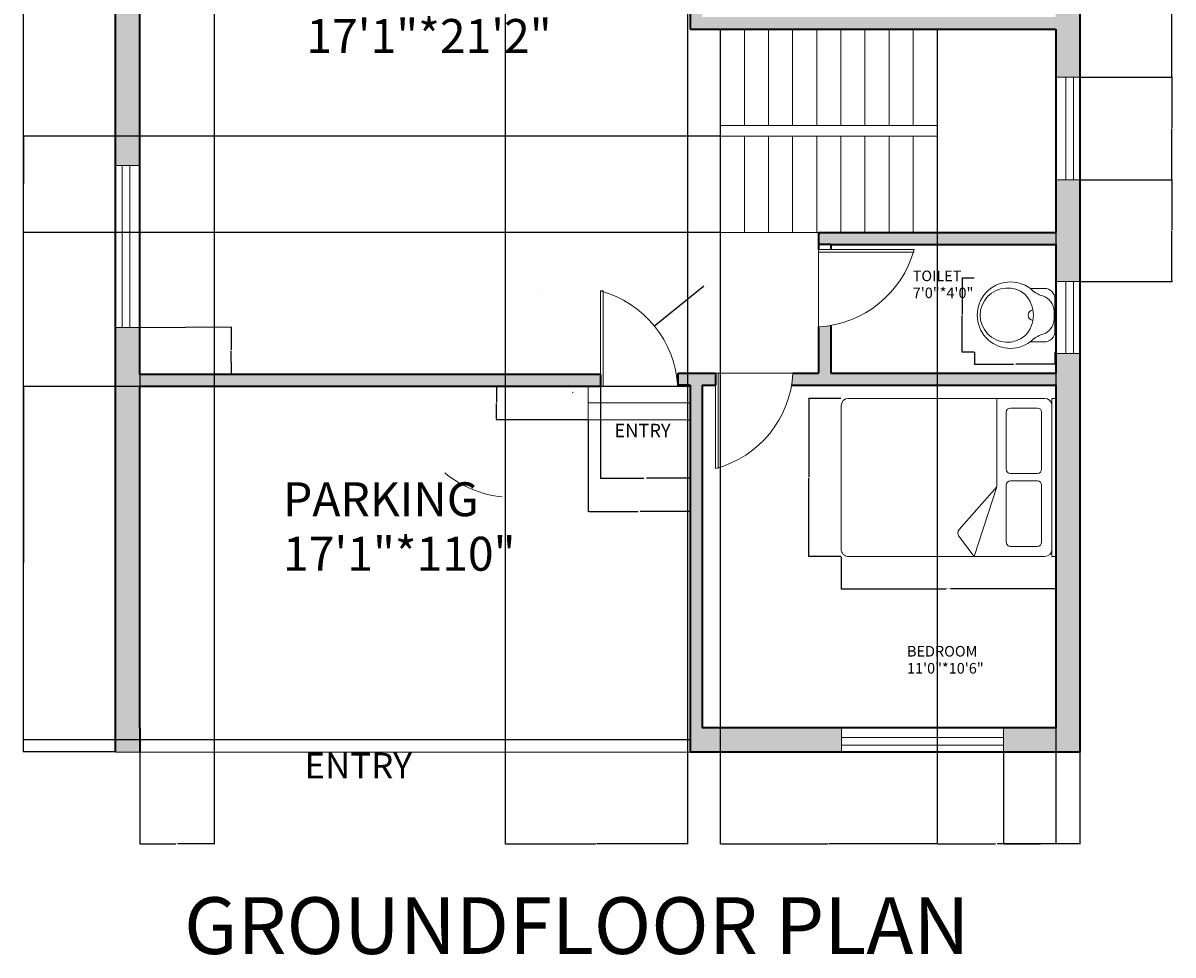
# Model space of a CAD drawing. Units: feet. Extents: x 2516 to 2945, y 1283 to 1993.
# Tile 1 of 3: x 2516 to 2945, y 1283 to 1631. Entities that reach past the tile are written whole.
import ezdxf

# ---------------------------------------------------------------- set-up
doc = ezdxf.new("R2010")
doc.units = ezdxf.units.FT
doc.layers.get('0').update_dxf_attribs({"lineweight": 18})
for name, color, linetype, lineweight in [('A-ANNO-DIMS', 2, 'Continuous', 18), ('A-ANNO-TEXT', 7, 'Continuous', 18), ('A-AREA-IDEN', 7, 'Continuous', 18), ('A-FLOR', 221, 'Continuous', 18), ('A-FLOR-FIXT', 8, 'Continuous', 18), ('A-FLOR-STRS', 7, 'Continuous', 18), ('A-FURN', 8, 'Continuous', 18), ('A-WALL', 7, 'Continuous', 35), ('A-WALL-PATT', 143, 'Continuous', 13), ('doors', 163, 'Continuous', 18), ('windows', 10, 'Continuous', 18)]:
    doc.layers.add(name, color=color, linetype=linetype, lineweight=lineweight)
doc.styles.get("Standard").update_dxf_attribs({"font": 'arial.ttf'})
doc.dimstyles.get("Standard").update_dxf_attribs({"dimtxt": 0.18, "dimasz": 0.18, "dimexe": 0.18, "dimexo": 0.0625, "dimgap": 0.09, "dimtad": 0, "dimtih": 1, "dimtoh": 1, "dimdec": 4, "dimzin": 0, "dimdsep": 46, "dimtxsty": 'Standard', "dimcen": 0.09, "dimadec": 0, "dimazin": 0, "dimtfac": 1, "dimtdec": 4, "dimtofl": 0, "dimtmove": 0, "dimatfit": 3, "dimfxl": 1, "dimtolj": 1, "dimtzin": 0, "dimarcsym": 0})

# ---------------------------------------------------------------- blocks, each defined once
blk = doc.blocks.new('door')
at = {"layer": 'doors'}
for p, q in [((-0.98, 0), (-0.98, 35.67)), ((0, 35.67), (0, 0)), ((-0.98, 0), (27.91, 0))]:
    blk.add_line(p, q, dxfattribs=at)
blk.add_arc((-11.23, -2.17), 39.2, 3.167, 74.8469, dxfattribs=at)
blk = doc.blocks.new('A$C6EF51710')
at = {"linetype": 'ByBlock'}
for p, q in [((0.0508, 0.2843), (0.1169, 0.2843)), ((0, 0.0811), (0, 0.2335)), ((0.0041, 0.1392), (0.0041, 0.1755)), ((0.1169, 0.0303), (0.0508, 0.0303))]:
    blk.add_line(p, q, dxfattribs=at)
for centre, radius, start, end in [((0.0508, 0.2335), 0.0508, 90, 180), ((0.0168, 0.3818), 0.1397, 287.1046, 315), ((0.2107, 0.1573), 0.1576, 232.8984, 127.1016), ((0.2254, 0.1573), 0.1289, 230.0084, 129.9916), ((0.0803, 0.1755), 0.0762, 107.1046, 180), ((0.2413, 0.1573), 0.1397, 135, 225), ((0.1016, 0.1573), 0.0254, 275.2159, 84.7841), ((0.0803, 0.1392), 0.0762, 180, 252.8954), ((0.0508, 0.0811), 0.0508, 180, 270), ((0.0168, -0.0672), 0.1397, 45, 72.8954)]:
    blk.add_arc(centre, radius, start, end, dxfattribs=at)
blk = doc.blocks.new('A$C03A44EBA')
at = {"rotation": 270}
blk.add_blockref('A$C6EF51710', (0.0003, 0.3683), dxfattribs=at)
blk = doc.blocks.new('A$C164346CA')
for p, q in [((0, 2.035), (0, 2)), ((1.5, 2.035), (0, 2.035)), ((1.5, 2), (0, 2)), ((1.5, 2), (1.5, 2.035)), ((0, 1.93), (0, 0.07)), ((0.092, 1.862), (0.092, 1.607)), ((0.673, 1.902), (0.132, 1.902)), ((0.713, 1.607), (0.713, 1.862)), ((0.783, 1.862), (0.783, 1.607)), ((1.364, 1.902), (0.823, 1.902)), ((1.404, 1.607), (1.404, 1.862)), ((1.5, 0.07), (1.5, 1.93)), ((0.132, 1.567), (0.673, 1.567)), ((0.823, 1.567), (1.364, 1.567)), ((0.839, 1.476), (0, 1.476)), ((0.839, 1.476), (1.245, 1.12)), ((1.5, 1.261), (0.839, 1.476)), ((1.308, 1.117), (1.5, 1.261)), ((0.07, 0), (1.43, 0))]:
    blk.add_line(p, q)
for centre, radius, start, end in [((0.07, 1.93), 0.07, 90, 180), ((1.43, 1.93), 0.07, 0, 90), ((0.132, 1.862), 0.04, 90, 180), ((0.673, 1.862), 0.04, 0, 90), ((0.823, 1.862), 0.04, 90, 180), ((1.364, 1.862), 0.04, 0, 90), ((0.132, 1.607), 0.04, 180, 270), ((0.673, 1.607), 0.04, 270, 0), ((0.823, 1.607), 0.04, 180, 270), ((1.364, 1.607), 0.04, 270, 0), ((1.278, 1.158), 0.05, 228.6958, 306.7579), ((0.07, 0.07), 0.07, 180, 270), ((1.43, 0.07), 0.07, 270, 0)]:
    blk.add_arc(centre, radius, start, end)
blk = doc.blocks.new('WIN-STANDARD')
for p, q in [((2.52, 60.52), (2.52, 0)), ((5.4, 60.52), (5.4, 0))]:
    blk.add_line(p, q)
blk.add_lwpolyline([(0, 60.52), (9, 60.52), (9, 0), (0, 0)], close=True)
blk = doc.blocks.new('WIN-TOILET')
for p, q in [((0, 5.4), (26.87, 5.4)), ((0, 2.52), (26.87, 2.52))]:
    blk.add_line(p, q)
blk.add_lwpolyline([(0, 9), (26.87, 9), (26.87, 0), (0, 0)], close=True)
blk = doc.blocks.new('*D17')
at = {"layer": 'A-ANNO-DIMS', "color": 0, "lineweight": -2, "transparency": 16777216}
for p, q in [((2821.29, 1431.8), (2821.29, 1419.66)), ((2901.42, 1431.8), (2901.42, 1419.66)), ((2821.47, 1419.84), (2860.54, 1419.84)), ((2901.24, 1419.84), (2862.17, 1419.84))]:
    blk.add_line(p, q, dxfattribs=at)
at = {"layer": 'A-ANNO-DIMS', "color": 0, "transparency": 16777216}
for points in [[(2821.47, 1419.87), (2821.47, 1419.81), (2821.29, 1419.84)], [(2901.24, 1419.87), (2901.24, 1419.81), (2901.42, 1419.84)]]:
    blk.add_solid(points, dxfattribs=at)
at = {"layer": 'Defpoints', "color": 0, "transparency": 16777216}
for p in [(2821.29, 1431.86), (2901.42, 1431.86), (2901.42, 1419.84)]:
    blk.add_point(p, dxfattribs=at)
at = {"layer": 'A-ANNO-DIMS', "color": 0, "transparency": 16777216, "insert": (2861.36, 1419.84), "char_height": 0.18, "attachment_point": 5}
blk.add_mtext('\\A1;BED 80 TYP.', dxfattribs=at)
blk = doc.blocks.new('*D18')
at = {"layer": 'A-ANNO-DIMS', "color": 0, "lineweight": -2, "transparency": 16777216}
for p, q in [((2821.23, 1490.92), (2809.1, 1490.92)), ((2809.28, 1490.74), (2809.28, 1461.57)), ((2809.28, 1432.04), (2809.28, 1461.21)), ((2821.23, 1431.86), (2809.1, 1431.86))]:
    blk.add_line(p, q, dxfattribs=at)
at = {"layer": 'A-ANNO-DIMS', "color": 0, "transparency": 16777216}
for points in [[(2809.25, 1490.74), (2809.31, 1490.74), (2809.28, 1490.92)], [(2809.25, 1432.04), (2809.31, 1432.04), (2809.28, 1431.86)]]:
    blk.add_solid(points, dxfattribs=at)
at = {"layer": 'Defpoints', "color": 0, "transparency": 16777216}
for p in [(2821.29, 1490.92), (2809.28, 1431.86), (2821.29, 1431.86)]:
    blk.add_point(p, dxfattribs=at)
at = {"layer": 'A-ANNO-DIMS', "color": 0, "transparency": 16777216, "insert": (2809.28, 1461.39), "char_height": 0.18, "attachment_point": 5}
blk.add_mtext('\\A1;59 TYP.', dxfattribs=at)
blk = doc.blocks.new('*D21')
at = {"layer": 'A-ANNO-DIMS', "color": 0, "lineweight": -2, "transparency": 16777216}
for p, q in [((2871.05, 1508.18), (2871.05, 1503.55)), ((2901.12, 1508.18), (2901.12, 1503.55)), ((2871.23, 1503.73), (2885.62, 1503.73)), ((2900.94, 1503.73), (2886.55, 1503.73))]:
    blk.add_line(p, q, dxfattribs=at)
at = {"layer": 'A-ANNO-DIMS', "color": 0, "transparency": 16777216}
for points in [[(2871.23, 1503.76), (2871.23, 1503.7), (2871.05, 1503.73)], [(2900.94, 1503.76), (2900.94, 1503.7), (2901.12, 1503.73)]]:
    blk.add_solid(points, dxfattribs=at)
at = {"layer": 'Defpoints', "color": 0, "transparency": 16777216}
for p in [(2871.05, 1508.24), (2901.12, 1508.24), (2901.12, 1503.73)]:
    blk.add_point(p, dxfattribs=at)
at = {"layer": 'A-ANNO-DIMS', "color": 0, "transparency": 16777216, "insert": (2886.09, 1503.73), "char_height": 0.18, "attachment_point": 5}
blk.add_mtext('\\A1;WC 30', dxfattribs=at)
blk = doc.blocks.new('*D22')
at = {"layer": 'A-ANNO-DIMS', "color": 0, "lineweight": -2, "transparency": 16777216}
for p, q in [((2870.99, 1535.77), (2866.36, 1535.77)), ((2866.54, 1535.59), (2866.54, 1522.19)), ((2866.54, 1508.42), (2866.54, 1521.83)), ((2870.99, 1508.24), (2866.36, 1508.24))]:
    blk.add_line(p, q, dxfattribs=at)
at = {"layer": 'A-ANNO-DIMS', "color": 0, "transparency": 16777216}
for points in [[(2866.51, 1535.59), (2866.57, 1535.59), (2866.54, 1535.77)], [(2866.51, 1508.42), (2866.57, 1508.42), (2866.54, 1508.24)]]:
    blk.add_solid(points, dxfattribs=at)
at = {"layer": 'Defpoints', "color": 0, "transparency": 16777216}
for p in [(2871.05, 1535.77), (2866.54, 1508.24), (2871.05, 1508.24)]:
    blk.add_point(p, dxfattribs=at)
at = {"layer": 'A-ANNO-DIMS', "color": 0, "transparency": 16777216, "insert": (2866.54, 1522.01), "char_height": 0.18, "attachment_point": 5}
blk.add_mtext('\\A1;28', dxfattribs=at)
blk = doc.blocks.new('*D28')
at = {"layer": 'A-ANNO-DIMS', "color": 0, "lineweight": -2, "transparency": 16777216}
for p, q in [((2550.35, 1958.86), (2515.85, 1958.86)), ((2516.03, 1958.68), (2516.03, 1659.04)), ((2516.03, 1359.04), (2516.03, 1658.68)), ((2550.35, 1358.86), (2515.85, 1358.86))]:
    blk.add_line(p, q, dxfattribs=at)
at = {"layer": 'A-ANNO-DIMS', "color": 0, "transparency": 16777216}
for points in [[(2516, 1958.68), (2516.06, 1958.68), (2516.03, 1958.86)], [(2516, 1359.04), (2516.06, 1359.04), (2516.03, 1358.86)]]:
    blk.add_solid(points, dxfattribs=at)
at = {"layer": 'Defpoints', "color": 0, "transparency": 16777216}
for p in [(2516.03, 1958.86), (2550.42, 1958.86), (2550.42, 1358.86)]:
    blk.add_point(p, dxfattribs=at)
at = {"layer": 'A-ANNO-DIMS', "color": 0, "transparency": 16777216, "insert": (2516.03, 1658.86), "char_height": 0.18, "attachment_point": 5}
blk.add_mtext('\\A1;600', dxfattribs=at)
blk = doc.blocks.new('*D31')
at = {"layer": 'A-ANNO-DIMS', "color": 0, "lineweight": -2, "transparency": 16777216}
for p, q in [((2881.98, 1358.8), (2881.98, 1324.43)), ((2910.42, 1358.8), (2910.42, 1324.43)), ((2882.16, 1324.61), (2895.8, 1324.61)), ((2910.24, 1324.61), (2896.59, 1324.61))]:
    blk.add_line(p, q, dxfattribs=at)
at = {"layer": 'A-ANNO-DIMS', "color": 0, "transparency": 16777216}
for points in [[(2882.16, 1324.64), (2882.16, 1324.58), (2881.98, 1324.61)], [(2910.24, 1324.64), (2910.24, 1324.58), (2910.42, 1324.61)]]:
    blk.add_solid(points, dxfattribs=at)
at = {"layer": 'Defpoints', "color": 0, "transparency": 16777216}
for p in [(2881.98, 1358.86), (2910.42, 1358.86), (2910.42, 1324.61)]:
    blk.add_point(p, dxfattribs=at)
at = {"layer": 'A-ANNO-DIMS', "color": 0, "transparency": 16777216, "insert": (2896.2, 1324.61), "char_height": 0.18, "attachment_point": 5}
blk.add_mtext('\\A1;28.44', dxfattribs=at)
blk = doc.blocks.new('*D32')
at = {"layer": 'A-ANNO-DIMS', "color": 0, "lineweight": -2, "transparency": 16777216}
for p, q in [((2559.34, 1517.39), (2593.71, 1517.65)), ((2593.53, 1517.47), (2593.6, 1509.07)), ((2593.66, 1500.3), (2593.6, 1508.71)), ((2559.48, 1499.86), (2593.85, 1500.13))]:
    blk.add_line(p, q, dxfattribs=at)
at = {"layer": 'A-ANNO-DIMS', "color": 0, "transparency": 16777216}
for points in [[(2593.56, 1517.47), (2593.5, 1517.47), (2593.53, 1517.65)], [(2593.69, 1500.3), (2593.63, 1500.3), (2593.67, 1500.12)]]:
    blk.add_solid(points, dxfattribs=at)
at = {"layer": 'Defpoints', "color": 0, "transparency": 16777216}
for p in [(2559.28, 1517.39), (2559.42, 1499.86), (2593.67, 1500.12)]:
    blk.add_point(p, dxfattribs=at)
at = {"layer": 'A-ANNO-DIMS', "color": 0, "transparency": 16777216, "insert": (2593.6, 1508.89), "char_height": 0.18, "attachment_point": 5}
blk.add_mtext('\\A1;17.53', dxfattribs=at)
blk = doc.blocks.new('*D37')
at = {"layer": 'A-ANNO-DIMS', "color": 0, "lineweight": -2, "transparency": 16777216}
for p, q in [((2910.48, 1663.1), (2945.03, 1663.1)), ((2944.85, 1662.92), (2944.85, 1637.15)), ((2944.85, 1611.01), (2944.85, 1636.78)), ((2910.48, 1610.83), (2945.03, 1610.83))]:
    blk.add_line(p, q, dxfattribs=at)
at = {"layer": 'A-ANNO-DIMS', "color": 0, "transparency": 16777216}
for points in [[(2944.82, 1662.92), (2944.88, 1662.92), (2944.85, 1663.1)], [(2944.82, 1611.01), (2944.88, 1611.01), (2944.85, 1610.83)]]:
    blk.add_solid(points, dxfattribs=at)
at = {"layer": 'Defpoints', "color": 0, "transparency": 16777216}
for p in [(2910.42, 1663.1), (2944.85, 1663.1), (2910.42, 1610.83)]:
    blk.add_point(p, dxfattribs=at)
at = {"layer": 'A-ANNO-DIMS', "color": 0, "transparency": 16777216, "insert": (2944.85, 1636.97), "char_height": 0.18, "attachment_point": 5}
blk.add_mtext('\\A1;52.26', dxfattribs=at)
blk = doc.blocks.new('*D38')
at = {"layer": 'A-ANNO-DIMS', "color": 0, "lineweight": -2, "transparency": 16777216}
for p, q in [((2910.48, 1610.83), (2945.03, 1610.83)), ((2944.85, 1610.65), (2944.85, 1591.89)), ((2944.85, 1572.76), (2944.85, 1591.53)), ((2910.48, 1572.58), (2945.03, 1572.58))]:
    blk.add_line(p, q, dxfattribs=at)
at = {"layer": 'A-ANNO-DIMS', "color": 0, "transparency": 16777216}
for points in [[(2944.82, 1610.65), (2944.88, 1610.65), (2944.85, 1610.83)], [(2944.82, 1572.76), (2944.88, 1572.76), (2944.85, 1572.58)]]:
    blk.add_solid(points, dxfattribs=at)
at = {"layer": 'Defpoints', "color": 0, "transparency": 16777216}
for p in [(2910.42, 1610.83), (2944.85, 1610.83), (2910.42, 1572.58)]:
    blk.add_point(p, dxfattribs=at)
at = {"layer": 'A-ANNO-DIMS', "color": 0, "transparency": 16777216, "insert": (2944.85, 1591.71), "char_height": 0.18, "attachment_point": 5}
blk.add_mtext('\\A1;38.25', dxfattribs=at)
blk = doc.blocks.new('*D39')
at = {"layer": 'A-ANNO-DIMS', "color": 0, "lineweight": -2, "transparency": 16777216}
for p, q in [((2910.48, 1572.58), (2945.03, 1572.58)), ((2944.85, 1572.4), (2944.85, 1553.76)), ((2944.85, 1534.76), (2944.85, 1553.4)), ((2910.66, 1534.58), (2945.03, 1534.58))]:
    blk.add_line(p, q, dxfattribs=at)
at = {"layer": 'A-ANNO-DIMS', "color": 0, "transparency": 16777216}
for points in [[(2944.82, 1572.4), (2944.88, 1572.4), (2944.85, 1572.58)], [(2944.82, 1534.76), (2944.88, 1534.76), (2944.85, 1534.58)]]:
    blk.add_solid(points, dxfattribs=at)
at = {"layer": 'Defpoints', "color": 0, "transparency": 16777216}
for p in [(2910.42, 1572.58), (2944.85, 1572.58), (2910.6, 1534.58)]:
    blk.add_point(p, dxfattribs=at)
at = {"layer": 'A-ANNO-DIMS', "color": 0, "transparency": 16777216, "insert": (2944.85, 1553.58), "char_height": 0.18, "attachment_point": 5}
blk.add_mtext('\\A1;38.004', dxfattribs=at)
blk = doc.blocks.new('*D40')
at = {"layer": 'A-ANNO-DIMS', "color": 0, "lineweight": -2, "transparency": 16777216}
for p, q in [((2776.18, 1628.8), (2776.18, 1324.43)), ((2857.18, 1628.8), (2857.18, 1324.43)), ((2776.36, 1324.61), (2816.48, 1324.61)), ((2857, 1324.61), (2816.88, 1324.61))]:
    blk.add_line(p, q, dxfattribs=at)
at = {"layer": 'A-ANNO-DIMS', "color": 0, "transparency": 16777216}
for points in [[(2776.36, 1324.64), (2776.36, 1324.58), (2776.18, 1324.61)], [(2857, 1324.64), (2857, 1324.58), (2857.18, 1324.61)]]:
    blk.add_solid(points, dxfattribs=at)
at = {"layer": 'Defpoints', "color": 0, "transparency": 16777216}
for p in [(2776.18, 1628.86), (2857.18, 1628.86), (2857.18, 1324.61)]:
    blk.add_point(p, dxfattribs=at)
at = {"layer": 'A-ANNO-DIMS', "color": 0, "transparency": 16777216, "insert": (2816.68, 1324.61), "char_height": 0.18, "attachment_point": 5}
blk.add_mtext('\\A1;81', dxfattribs=at)
blk = doc.blocks.new('*D41')
at = {"layer": 'A-ANNO-DIMS', "color": 0, "lineweight": -2, "transparency": 16777216}
for p, q in [((2857.18, 1628.8), (2857.18, 1324.43)), ((2901.42, 1628.8), (2901.42, 1324.43)), ((2857.36, 1324.61), (2878.9, 1324.61)), ((2901.24, 1324.61), (2879.7, 1324.61))]:
    blk.add_line(p, q, dxfattribs=at)
at = {"layer": 'A-ANNO-DIMS', "color": 0, "transparency": 16777216}
for points in [[(2857.36, 1324.64), (2857.36, 1324.58), (2857.18, 1324.61)], [(2901.24, 1324.64), (2901.24, 1324.58), (2901.42, 1324.61)]]:
    blk.add_solid(points, dxfattribs=at)
at = {"layer": 'Defpoints', "color": 0, "transparency": 16777216}
for p in [(2857.18, 1628.86), (2901.42, 1628.86), (2901.42, 1324.61)]:
    blk.add_point(p, dxfattribs=at)
at = {"layer": 'A-ANNO-DIMS', "color": 0, "transparency": 16777216, "insert": (2879.3, 1324.61), "char_height": 0.18, "attachment_point": 5}
blk.add_mtext('\\A1;44.24', dxfattribs=at)
blk = doc.blocks.new('*D42')
at = {"layer": 'A-ANNO-DIMS', "color": 0, "lineweight": -2, "transparency": 16777216}
for p, q in [((2776.12, 1588.86), (2515.85, 1588.86)), ((2516.03, 1588.68), (2516.03, 1571.04)), ((2516.03, 1553.04), (2516.03, 1570.68)), ((2776.12, 1552.86), (2515.85, 1552.86))]:
    blk.add_line(p, q, dxfattribs=at)
at = {"layer": 'A-ANNO-DIMS', "color": 0, "transparency": 16777216}
for points in [[(2516, 1588.68), (2516.06, 1588.68), (2516.03, 1588.86)], [(2516, 1553.04), (2516.06, 1553.04), (2516.03, 1552.86)]]:
    blk.add_solid(points, dxfattribs=at)
at = {"layer": 'Defpoints', "color": 0, "transparency": 16777216}
for p in [(2516.03, 1588.86), (2776.18, 1588.86), (2776.18, 1552.86)]:
    blk.add_point(p, dxfattribs=at)
at = {"layer": 'A-ANNO-DIMS', "color": 0, "transparency": 16777216, "insert": (2516.03, 1570.86), "char_height": 0.18, "attachment_point": 5}
blk.add_mtext('\\A1;36', dxfattribs=at)
blk = doc.blocks.new('*D43')
at = {"layer": 'A-ANNO-DIMS', "color": 0, "lineweight": -2, "transparency": 16777216}
for p, q in [((2695.92, 1802.8), (2695.92, 1324.43)), ((2763.92, 1802.8), (2763.92, 1324.43)), ((2696.1, 1324.61), (2729.7, 1324.61)), ((2763.74, 1324.61), (2730.14, 1324.61))]:
    blk.add_line(p, q, dxfattribs=at)
at = {"layer": 'A-ANNO-DIMS', "color": 0, "transparency": 16777216}
for points in [[(2696.1, 1324.64), (2696.1, 1324.58), (2695.92, 1324.61)], [(2763.74, 1324.64), (2763.74, 1324.58), (2763.92, 1324.61)]]:
    blk.add_solid(points, dxfattribs=at)
at = {"layer": 'Defpoints', "color": 0, "transparency": 16777216}
for p in [(2695.92, 1802.86), (2763.92, 1802.86), (2763.92, 1324.61)]:
    blk.add_point(p, dxfattribs=at)
at = {"layer": 'A-ANNO-DIMS', "color": 0, "transparency": 16777216, "insert": (2729.92, 1324.61), "char_height": 0.18, "attachment_point": 5}
blk.add_mtext('\\A1;68', dxfattribs=at)
blk = doc.blocks.new('*D45')
at = {"layer": 'A-ANNO-DIMS', "color": 0, "lineweight": -2, "transparency": 16777216}
for p, q in [((2764.85, 1495.36), (2515.85, 1495.36)), ((2516.03, 1495.18), (2516.03, 1429.54)), ((2516.03, 1363.54), (2516.03, 1429.18)), ((2764.85, 1363.36), (2515.85, 1363.36))]:
    blk.add_line(p, q, dxfattribs=at)
at = {"layer": 'A-ANNO-DIMS', "color": 0, "transparency": 16777216}
for points in [[(2516, 1495.18), (2516.06, 1495.18), (2516.03, 1495.36)], [(2516, 1363.54), (2516.06, 1363.54), (2516.03, 1363.36)]]:
    blk.add_solid(points, dxfattribs=at)
at = {"layer": 'Defpoints', "color": 0, "transparency": 16777216}
for p in [(2516.03, 1495.36), (2764.92, 1495.36), (2764.92, 1363.36)]:
    blk.add_point(p, dxfattribs=at)
at = {"layer": 'A-ANNO-DIMS', "color": 0, "transparency": 16777216, "insert": (2516.03, 1429.36), "char_height": 0.18, "attachment_point": 5}
blk.add_mtext('\\A1;132', dxfattribs=at)
blk = doc.blocks.new('*D46')
at = {"layer": 'A-ANNO-DIMS', "color": 0, "lineweight": -2, "transparency": 16777216}
for p, q in [((2559.42, 1870.95), (2559.42, 1324.43)), ((2587.15, 1870.95), (2587.15, 1324.43)), ((2559.6, 1324.61), (2572.89, 1324.61)), ((2586.97, 1324.61), (2573.68, 1324.61))]:
    blk.add_line(p, q, dxfattribs=at)
at = {"layer": 'A-ANNO-DIMS', "color": 0, "transparency": 16777216}
for points in [[(2559.6, 1324.64), (2559.6, 1324.58), (2559.42, 1324.61)], [(2586.97, 1324.64), (2586.97, 1324.58), (2587.15, 1324.61)]]:
    blk.add_solid(points, dxfattribs=at)
at = {"layer": 'Defpoints', "color": 0, "transparency": 16777216}
for p in [(2559.42, 1871.01), (2587.15, 1871.01), (2587.15, 1324.61)]:
    blk.add_point(p, dxfattribs=at)
at = {"layer": 'A-ANNO-DIMS', "color": 0, "transparency": 16777216, "insert": (2573.29, 1324.61), "char_height": 0.18, "attachment_point": 5}
blk.add_mtext('\\A1;27.74', dxfattribs=at)
blk = doc.blocks.new('*D48')
at = {"layer": 'A-ANNO-DIMS', "color": 0, "lineweight": -2, "transparency": 16777216}
for p, q in [((2731.41, 1495.3), (2731.41, 1460.93)), ((2764.92, 1495.3), (2764.92, 1460.93)), ((2731.59, 1461.11), (2747.7, 1461.11)), ((2764.74, 1461.11), (2748.63, 1461.11))]:
    blk.add_line(p, q, dxfattribs=at)
at = {"layer": 'A-ANNO-DIMS', "color": 0, "transparency": 16777216}
for points in [[(2731.59, 1461.14), (2731.59, 1461.08), (2731.41, 1461.11)], [(2764.74, 1461.14), (2764.74, 1461.08), (2764.92, 1461.11)]]:
    blk.add_solid(points, dxfattribs=at)
at = {"layer": 'Defpoints', "color": 0, "transparency": 16777216}
for p in [(2731.41, 1495.36), (2764.92, 1495.36), (2731.41, 1461.11)]:
    blk.add_point(p, dxfattribs=at)
at = {"layer": 'A-ANNO-DIMS', "color": 0, "transparency": 16777216, "insert": (2748.16, 1461.11), "char_height": 0.18, "attachment_point": 5}
blk.add_mtext('\\A1;33.507', dxfattribs=at)
blk = doc.blocks.new('*D52')
at = {"layer": 'A-ANNO-DIMS', "color": 0, "lineweight": -2, "transparency": 16777216}
for p, q in [((2726.81, 1495.36), (2692.44, 1495.36)), ((2692.62, 1495.18), (2692.62, 1489.33)), ((2692.62, 1483.13), (2692.62, 1488.97)), ((2726.81, 1482.95), (2692.44, 1482.95))]:
    blk.add_line(p, q, dxfattribs=at)
at = {"layer": 'A-ANNO-DIMS', "color": 0, "transparency": 16777216}
for points in [[(2692.59, 1495.18), (2692.65, 1495.18), (2692.62, 1495.36)], [(2692.59, 1483.13), (2692.65, 1483.13), (2692.62, 1482.95)]]:
    blk.add_solid(points, dxfattribs=at)
at = {"layer": 'Defpoints', "color": 0, "transparency": 16777216}
for p in [(2692.62, 1495.36), (2726.87, 1495.36), (2726.87, 1482.95)]:
    blk.add_point(p, dxfattribs=at)
at = {"layer": 'A-ANNO-DIMS', "color": 0, "transparency": 16777216, "insert": (2692.62, 1489.15), "char_height": 0.18, "attachment_point": 5}
blk.add_mtext('\\A1;12.41', dxfattribs=at)
blk = doc.blocks.new('*D53')
at = {"layer": 'A-ANNO-DIMS', "color": 0, "lineweight": -2, "transparency": 16777216}
for p, q in [((2726.87, 1482.89), (2726.87, 1448.52)), ((2764.92, 1482.89), (2764.92, 1448.52)), ((2727.05, 1448.7), (2745.5, 1448.7)), ((2764.74, 1448.7), (2746.29, 1448.7))]:
    blk.add_line(p, q, dxfattribs=at)
at = {"layer": 'A-ANNO-DIMS', "color": 0, "transparency": 16777216}
for points in [[(2727.05, 1448.73), (2727.05, 1448.67), (2726.87, 1448.7)], [(2764.74, 1448.73), (2764.74, 1448.67), (2764.92, 1448.7)]]:
    blk.add_solid(points, dxfattribs=at)
at = {"layer": 'Defpoints', "color": 0, "transparency": 16777216}
for p in [(2726.87, 1482.95), (2764.92, 1482.95), (2726.87, 1448.7)]:
    blk.add_point(p, dxfattribs=at)
at = {"layer": 'A-ANNO-DIMS', "color": 0, "transparency": 16777216, "insert": (2745.89, 1448.7), "char_height": 0.18, "attachment_point": 5}
blk.add_mtext('\\A1;38.05', dxfattribs=at)
blk = doc.blocks.new('*D54')
at = {"layer": 'A-ANNO-DIMS', "color": 0, "lineweight": -2, "transparency": 16777216}
for p, q in [((2769.9, 1532.67), (2751.76, 1517.98)), ((2770.08, 1532.67), (2769.9, 1532.67)), ((2721.07, 1493.19), (2721.25, 1493.19)), ((2721.16, 1493.1), (2721.16, 1493.28))]:
    blk.add_line(p, q, dxfattribs=at)
at = {"layer": 'A-ANNO-DIMS', "color": 0, "transparency": 16777216}
blk.add_solid([(2751.74, 1518), (2751.78, 1517.95), (2751.62, 1517.86)], dxfattribs=at)
at = {"layer": 'Defpoints', "color": 0, "transparency": 16777216}
for p in [(2751.62, 1517.86), (2721.16, 1493.19)]:
    blk.add_point(p, dxfattribs=at)
at = {"layer": 'A-ANNO-DIMS', "color": 0, "transparency": 16777216, "insert": (2770.69, 1532.67), "char_height": 0.18, "attachment_point": 5}
blk.add_mtext('\\A1;4X R39.2', dxfattribs=at)

msp = doc.modelspace()

# ---------------------------------------------------------------- hatches: boundary and pattern name
at = {"layer": 'A-WALL-PATT'}
h = msp.add_hatch(color=256, dxfattribs=at)
h.dxf.hatch_style = 1
h.paths.add_polyline_path([(2763.9169, 1832.358), (2695.9169, 1832.358), (2695.9169, 1845.8137), (2691.4169, 1845.8137), (2691.4169, 1802.858), (2695.9169, 1802.858), (2695.9169, 1827.858), (2763.9169, 1827.858)])
h.paths.add_polyline_path([(2768.4169, 1886.6758), (2763.9169, 1886.6758), (2763.9169, 1789.8455), (2764.9169, 1789.8455), (2764.9169, 1790.0678, -0.01619533), (2767.4458, 1789.8455), (2768.4169, 1789.8455)])
h.paths.add_polyline_path([(2710.0911, 1958.858), (2663.1874, 1958.858), (2663.1874, 1949.858), (2691.4169, 1949.858), (2691.4169, 1878.358), (2763.9169, 1878.358), (2763.9169, 1882.858), (2695.9169, 1882.858), (2695.9169, 1949.858), (2710.0911, 1949.858)])
h.paths.add_polyline_path([(2910.4169, 1958.858), (2736.9631, 1958.858), (2736.9631, 1949.858), (2763.9169, 1949.858), (2763.9169, 1915.057, -0.02890868), (2768.4169, 1915.568), (2768.4169, 1949.858), (2901.4169, 1949.858), (2901.4169, 1859.2593), (2910.4169, 1859.2593)])
h.paths.add_polyline_path([(2910.4169, 1798.7389), (2901.4169, 1798.7389), (2901.4169, 1757.858), (2769.4169, 1757.858), (2769.4169, 1761.1755), (2764.9169, 1761.1755), (2764.9596, 1666.1291, -0.0286323), (2769.4169, 1665.6254), (2769.4169, 1753.358), (2901.4169, 1753.358), (2901.4169, 1723.6182), (2910.4169, 1723.6182)])
h.paths.add_polyline_path([(2910.4169, 1663.0978), (2901.4169, 1663.0978), (2901.4169, 1633.358), (2769.4169, 1633.358), (2769.4169, 1637.2369), (2764.9596, 1637.2369), (2764.9596, 1628.858), (2901.4169, 1628.858), (2901.4169, 1610.8331), (2910.4169, 1610.8331)])
h.paths.add_polyline_path([(2910.4169, 1572.5822), (2901.4169, 1572.5822), (2901.4169, 1552.858), (2812.9169, 1552.858), (2812.9169, 1548.358), (2817.4169, 1548.358), (2901.4169, 1548.358), (2901.4169, 1534.5783), (2910.4169, 1534.5783)])
h.paths.add_polyline_path([(2910.4169, 1507.7063), (2901.4169, 1507.7063), (2901.4169, 1500.358), (2817.4169, 1500.358), (2817.4169, 1518.131, -0.02890927), (2812.9169, 1517.6191), (2812.9169, 1500.358), (2803.3072, 1500.358, -0.02890868), (2802.7962, 1495.858), (2901.4169, 1495.858), (2901.4169, 1367.858), (2881.9751, 1367.858), (2881.9751, 1358.858), (2910.4169, 1358.858)])
h.paths.add_polyline_path([(2821.4547, 1367.858), (2769.4169, 1367.858), (2769.4169, 1495.858), (2774.415, 1495.858), (2774.415, 1500.358), (2760.4256, 1500.358), (2760.4256, 1495.858), (2764.9169, 1495.858), (2764.9169, 1367.858), (2764.9169, 1358.858), (2821.4547, 1358.858)])
h.paths.add_polyline_path([(2731.4104, 1499.858), (2559.4169, 1499.858), (2559.4169, 1495.358), (2731.4104, 1495.358)])
h.paths.add_polyline_path([(2559.4169, 1665.5276), (2550.4169, 1665.5276), (2550.4169, 1577.9069), (2559.4169, 1577.9069)])
h.paths.add_polyline_path([(2559.4169, 1767.1637), (2550.4169, 1767.1637), (2550.4169, 1726.0479), (2559.4169, 1726.0479)])
h.paths.add_polyline_path([(2695.9169, 1757.858), (2559.4169, 1757.858), (2559.4169, 1753.358), (2695.9169, 1753.358)])
h.paths.add_polyline_path([(2559.4169, 1949.858), (2602.667, 1949.858), (2602.667, 1958.858), (2550.4169, 1958.858), (2550.4169, 1827.6841), (2559.4169, 1827.6841)])
h = msp.add_hatch(color=256, dxfattribs=at)
h.dxf.hatch_style = 1
h.paths.add_polyline_path([(2559.4169, 1495.358), (2731.4104, 1495.358), (2731.4104, 1499.858), (2559.4169, 1499.858), (2559.4169, 1517.3865), (2550.4169, 1517.3865), (2550.4169, 1358.858), (2559.4169, 1358.858), (2559.4169, 1367.858)])

# ---------------------------------------------------------------- linework, layer by layer
at = {"layer": 'A-FLOR'}
for p, q in [((2559.4169, 1363.358), (2764.9169, 1363.358)), ((2550.4169, 1358.858), (2764.9169, 1358.858))]:
    msp.add_line(p, q, dxfattribs=at)
at = {"layer": 'A-FLOR-STRS'}
for p, q in [((2776.1811, 1628.858), (2776.1811, 1552.858)), ((2785.1811, 1628.858), (2785.1811, 1592.858)), ((2794.1811, 1628.858), (2794.1811, 1592.858)), ((2803.1811, 1628.858), (2803.1811, 1592.858)), ((2812.1811, 1628.858), (2812.1811, 1592.858)), ((2821.1811, 1628.858), (2821.1811, 1592.858)), ((2830.1811, 1628.858), (2830.1811, 1592.858)), ((2839.1811, 1628.858), (2839.1811, 1592.858)), ((2848.1811, 1628.858), (2848.1811, 1592.858)), ((2857.1811, 1628.858), (2857.1811, 1552.858)), ((2776.1811, 1592.858), (2857.1811, 1592.858)), ((2812.9169, 1588.858), (2776.1811, 1588.858)), ((2785.1811, 1588.858), (2785.1811, 1552.858)), ((2794.1811, 1588.858), (2794.1811, 1552.858)), ((2803.1811, 1588.858), (2803.1811, 1552.858)), ((2812.1811, 1588.858), (2812.1811, 1552.858)), ((2812.9169, 1588.858), (2857.1811, 1588.858)), ((2821.1811, 1588.858), (2821.1811, 1552.858)), ((2830.1811, 1588.858), (2830.1811, 1552.858)), ((2839.1811, 1588.858), (2839.1811, 1552.858)), ((2848.1811, 1588.858), (2848.1811, 1552.858)), ((2812.9169, 1552.858), (2776.1811, 1552.858))]:
    msp.add_line(p, q, dxfattribs=at)
for points in [[(2726.8685, 1495.358), (2764.9169, 1495.358), (2764.9169, 1489.2538), (2726.8685, 1489.2538)], [(2726.8685, 1489.2538), (2764.9169, 1489.2538), (2764.9169, 1482.9476), (2726.8685, 1482.9476)]]:
    msp.add_lwpolyline(points, close=True, dxfattribs=at)
at = {"layer": 'A-WALL'}
for p, q in [((2550.4169, 1358.858), (2550.4169, 1958.858)), ((2910.4169, 1958.858), (2910.4169, 1358.858)), ((2559.4169, 1499.858), (2559.4169, 1949.858)), ((2764.9596, 1637.2369), (2764.9596, 1628.858)), ((2764.9169, 1628.858), (2901.4169, 1628.858)), ((2901.4169, 1628.858), (2901.4169, 1552.858)), ((2812.9169, 1552.858), (2901.4169, 1552.858)), ((2812.9169, 1552.858), (2812.9169, 1546.5109)), ((2817.4169, 1548.358), (2812.9169, 1548.358)), ((2817.4169, 1548.358), (2901.4169, 1548.358)), ((2817.4169, 1548.358), (2817.4169, 1546.5109)), ((2901.4169, 1548.358), (2901.4169, 1500.358)), ((2812.9169, 1517.6191), (2812.9169, 1500.358)), ((2817.4169, 1518.131), (2817.4169, 1500.358)), ((2731.4104, 1499.858), (2559.4169, 1499.858)), ((2731.4104, 1499.858), (2731.4104, 1495.358)), ((2760.4256, 1495.858), (2760.4256, 1500.358)), ((2760.4256, 1500.358), (2774.415, 1500.358)), ((2774.415, 1500.358), (2774.415, 1495.858)), ((2803.3072, 1500.358), (2812.9169, 1500.358)), ((2817.4169, 1500.358), (2901.4169, 1500.358)), ((2559.4169, 1367.858), (2559.4169, 1495.358)), ((2731.4104, 1495.358), (2559.4169, 1495.358)), ((2764.9169, 1495.858), (2760.4256, 1495.858)), ((2764.9169, 1495.858), (2764.9169, 1367.858)), ((2769.4169, 1495.858), (2769.4169, 1367.858)), ((2769.4169, 1495.858), (2774.415, 1495.858)), ((2802.7962, 1495.858), (2901.4169, 1495.858)), ((2901.4169, 1495.858), (2901.4169, 1367.858)), ((2559.4169, 1367.858), (2559.4169, 1358.858)), ((2764.9169, 1367.858), (2764.9169, 1358.858)), ((2901.4169, 1367.858), (2769.4169, 1367.858)), ((2910.4169, 1358.858), (2764.9169, 1358.858))]:
    msp.add_line(p, q, dxfattribs=at)
at = {"layer": 'doors'}
for p, q in [((2708.6924, 1531.028), (2708.6924, 1531.028)), ((2731.4104, 1495.358), (2731.4104, 1531.028)), ((2731.4104, 1531.028), (2731.4104, 1531.028)), ((2731.4104, 1531.028), (2732.393, 1531.028)), ((2732.393, 1531.028), (2732.393, 1495.358)), ((2732.393, 1495.358), (2731.4104, 1495.358)), ((2731.4104, 1495.358), (2760.3026, 1495.358))]:
    msp.add_line(p, q, dxfattribs=at)
for centre, start, end in [((2721.1639, 1493.1924), 3.167032, 74.846949), ((2698.446, 1493.1924), 230.206563, 264.587023)]:
    msp.add_arc(centre, 39.1985, start, end, dxfattribs=at)
at = {"layer": 'windows'}
for p, q in [((2905.2031, 1572.5822), (2905.2031, 1610.8331)), ((2908.0795, 1572.5822), (2908.0795, 1610.8331))]:
    msp.add_line(p, q, dxfattribs=at)
msp.add_lwpolyline([(2901.4169, 1610.8331), (2910.4169, 1610.8331), (2910.4169, 1572.5822), (2901.4169, 1572.5822)], close=True, dxfattribs=at)

# ---------------------------------------------------------------- block references
at = {"layer": 'A-FLOR-FIXT', "xscale": 78.71591991659332, "yscale": 78.71591991659332, "zscale": 78.71591991659332, "rotation": 270.0000000000002}
msp.add_blockref('A$C03A44EBA', (2872.1301, 1534.4142), dxfattribs=at)
at = {"layer": 'A-FURN', "xscale": 39.37235568073177, "yscale": 39.37235568073177, "zscale": 39.37235568073177, "rotation": 269.9999999999978}
msp.add_blockref('A$C164346CA', (2821.2942, 1490.9165), dxfattribs=at)
at = {"layer": 'doors', "rotation": 270}
msp.add_blockref('door', (2812.91, 1545.5284), dxfattribs=at)
at = {"layer": 'doors', "xscale": -1, "rotation": 180}
msp.add_blockref('door', (2775.3976, 1500.358), dxfattribs=at)
at = {"layer": 'windows'}
msp.add_blockref('WIN-STANDARD', (2550.2809, 1517.3869), dxfattribs=at)
for name, p, rotation in [('WIN-TOILET', (2910.5987, 1507.7062), 90.0000000000013), ('WIN-STANDARD', (2881.9747, 1358.8581), 89.99999999999785)]:
    msp.add_blockref(name, p, dxfattribs=dict(at, rotation=rotation))

# ---------------------------------------------------------------- texts
at = {"layer": 'A-ANNO-TEXT'}
for s, height, p in [('ENTRY', 5.00139, (2736.6516, 1476.426)), ('ENTRY', 9.54526, (2620.9424, 1349.0158)), ('GROUNDFLOOR PLAN', 21.190169, (2575.9522, 1283.4226))]:
    msp.add_text(s, height=height, dxfattribs=at).set_placement(p)
at = {"layer": 'A-AREA-IDEN'}
for s, height, p in [('17\'1"*21\'2"', 12.669464, (2621.6224, 1619.9228)), ('TOILET', 3.95825, (2848.0501, 1534.6892)), ('7\'0"*4\'0"', 3.95825, (2848.0501, 1528.3306)), ('PARKING', 12.66946, (2612.9157, 1446.9135)), ('17\'1"*110"', 12.66946, (2612.9157, 1426.5611)), ('BEDROOM', 3.95825, (2845.9076, 1394.5006)), ('11\'0"*10\'6"', 3.958252, (2845.9076, 1388.142))]:
    msp.add_text(s, height=height, dxfattribs=at).set_placement(p)

# ---------------------------------------------------------------- dimensions: what is measured, and where the dimension line sits
at = {"layer": 'A-ANNO-DIMS'}
for base, p1, p2, angle, override, picture, middle in [((2516.0308, 1958.858), (2550.4169, 1358.858), (2550.4169, 1958.858), 90, {"dimdec": 0, "dimlfac": 1, "dimrnd": 0, "dimzin": 0, "dimdsep": 46, "dimlunit": 2}, '*D28', (2516.0308, 1658.858)), ((2944.8487, 1663.0978), (2910.4169, 1610.8331), (2910.4169, 1663.0978), 90, {"dimdec": 2, "dimlfac": 1, "dimrnd": 0, "dimzin": 0, "dimdsep": 46, "dimlunit": 2}, '*D37', (2944.8487, 1636.9654)), ((2944.8487, 1610.8331), (2910.4169, 1572.5822), (2910.4169, 1610.8331), 90, {"dimdec": 2, "dimlfac": 1, "dimrnd": 0, "dimzin": 0, "dimdsep": 46, "dimlunit": 2}, '*D38', (2944.8487, 1591.7076)), ((2516.0308, 1588.858), (2776.1811, 1552.858), (2776.1811, 1588.858), 90, {"dimdec": 0, "dimlfac": 1, "dimrnd": 0, "dimzin": 0, "dimdsep": 46, "dimlunit": 2}, '*D42', (2516.0308, 1570.858)), ((2944.8487, 1572.5822), (2910.5987, 1534.5783), (2910.4169, 1572.5822), 90, {"dimdec": 3, "dimlfac": 1, "dimrnd": 0, "dimzin": 0, "dimdsep": 46, "dimlunit": 2}, '*D39', (2944.8487, 1553.5802)), ((2866.5392, 1508.2429), (2871.0499, 1535.7713), (2871.0499, 1508.2429), 270, {"dimdec": 0, "dimlfac": 1, "dimrnd": 0, "dimzin": 0, "dimdsep": 46, "dimlunit": 2}, '*D22', (2866.5392, 1522.0071)), ((2593.6659, 1500.124), (2559.2808, 1517.3865), (2559.4169, 1499.858), 270.445003, {"dimdec": 2, "dimlfac": 1, "dimrnd": 0, "dimzin": 0, "dimdsep": 46, "dimlunit": 2}, '*D32', (2593.5978, 1508.8883)), ((2516.0308, 1495.358), (2764.9169, 1363.358), (2764.9169, 1495.358), 90, {"dimdec": 0, "dimlfac": 1, "dimrnd": 0, "dimzin": 0, "dimdsep": 46, "dimlunit": 2}, '*D45', (2516.0308, 1429.358)), ((2692.6185, 1495.358), (2726.8685, 1482.9476), (2726.8685, 1495.358), 90, {"dimdec": 2, "dimlfac": 1, "dimrnd": 0, "dimzin": 0, "dimdsep": 46, "dimlunit": 2}, '*D52', (2692.6185, 1489.1528)), ((2731.41037, 1461.108), (2764.91693, 1495.358), (2731.41037, 1495.358), 180, {"dimdec": 3, "dimlfac": 1, "dimrnd": 0, "dimzin": 0, "dimdsep": 46, "dimlunit": 2}, '*D48', (2748.16365, 1461.108)), ((2726.8685, 1448.6976), (2764.9169, 1482.9476), (2726.8685, 1482.9476), 180, {"dimdec": 2, "dimlfac": 1, "dimrnd": 0, "dimzin": 0, "dimdsep": 46, "dimlunit": 2}, '*D53', (2745.8927, 1448.6976))]:
    dim = msp.add_linear_dim(base=base, p1=p1, p2=p2, angle=angle, dimstyle='Standard', override=override, dxfattribs=at)
    dim.commit()
    dim.dimension.update_dxf_attribs({"geometry": picture, "text_midpoint": middle})
for base, p1, p2, override, picture, middle in [((2587.155, 1324.608), (2559.4169, 1871.0142), (2587.155, 1871.0142), {"dimdec": 2, "dimlfac": 1, "dimrnd": 0, "dimzin": 0, "dimdsep": 46, "dimlunit": 2}, '*D46', (2573.2859, 1324.608)), ((2763.9169, 1324.608), (2695.9169, 1802.858), (2763.9169, 1802.858), {"dimdec": 0, "dimlfac": 1, "dimrnd": 0, "dimzin": 0, "dimdsep": 46, "dimlunit": 2}, '*D43', (2729.9169, 1324.608)), ((2857.1811, 1324.608), (2776.1811, 1628.858), (2857.1811, 1628.858), {"dimdec": 0, "dimlfac": 1, "dimrnd": 0, "dimzin": 0, "dimdsep": 46, "dimlunit": 2}, '*D40', (2816.6811, 1324.608)), ((2901.4169, 1324.608), (2857.1811, 1628.858), (2901.4169, 1628.858), {"dimdec": 2, "dimlfac": 1, "dimrnd": 0, "dimzin": 0, "dimdsep": 46, "dimlunit": 2}, '*D41', (2879.299, 1324.608)), ((2910.4169, 1324.608), (2881.9751, 1358.858), (2910.4169, 1358.858), {"dimdec": 2, "dimlfac": 1, "dimrnd": 0, "dimzin": 0, "dimdsep": 46, "dimlunit": 2}, '*D31', (2896.196, 1324.608))]:
    dim = msp.add_linear_dim(base=base, p1=p1, p2=p2, dimstyle='Standard', override=override, dxfattribs=at)
    dim.commit()
    dim.dimension.update_dxf_attribs({"geometry": picture, "text_midpoint": middle})
dim = msp.add_radius_dim(center=(2721.1639, 1493.1924), mpoint=(2751.6237, 1517.8648), text='4X <>', dimstyle='Standard', override={"dimdec": 1, "dimlfac": 1, "dimrnd": 0, "dimzin": 0, "dimdsep": 46, "dimlunit": 2}, dxfattribs=at)
dim.commit()
dim.dimension.update_dxf_attribs({"geometry": '*D54', "text_midpoint": (2770.6856, 1532.6682), "dimtype": 164})
for base, p1, p2, angle, text, picture, middle in [((2901.1211, 1503.7322), (2871.0499, 1508.2429), (2901.1211, 1508.2429), 0, 'WC <>', '*D21', (2886.0855, 1503.7322)), ((2809.2758, 1431.858), (2821.2942, 1490.9165), (2821.2942, 1431.858), 270, '<> TYP.', '*D18', (2809.2758, 1461.3873))]:
    dim = msp.add_linear_dim(base=base, p1=p1, p2=p2, angle=angle, text=text, dimstyle='Standard', override={"dimdec": 0, "dimlfac": 1, "dimrnd": 0, "dimzin": 0, "dimdsep": 46, "dimlunit": 2}, dxfattribs=at)
    dim.commit()
    dim.dimension.update_dxf_attribs({"geometry": picture, "text_midpoint": middle})
dim = msp.add_linear_dim(base=(2901.4169, 1419.8396), p1=(2821.2942, 1431.858), p2=(2901.4169, 1431.858), text='BED <> TYP.', dimstyle='Standard', override={"dimdec": 0, "dimlfac": 1, "dimrnd": 0, "dimzin": 0, "dimdsep": 46, "dimlunit": 2}, dxfattribs=at)
dim.commit()
dim.dimension.update_dxf_attribs({"geometry": '*D17', "text_midpoint": (2861.3556, 1419.8396)})

doc.saveas('drawing.dxf')
